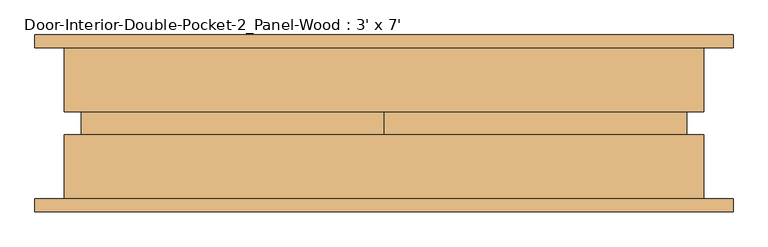
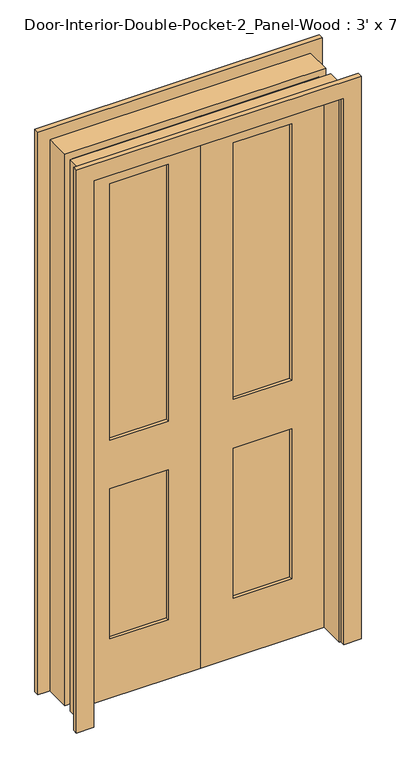
"""IFC4 building model written with IfcOpenShell, lengths in millimetres: door geometry, Door-Interior-Double-Pocket-2_Panel-Wood : 3' x 7'."""

from ifc_helpers import new_model, si_unit, frame, origin, place, context, project, spatial, polyline, outline, extrude, source, transform, mapped, element, save


def door_interior_double_pocket_2_panel_wood_3_x_7_65f9ecc5(model_context):
    return source(origin(), model_context, "Body", "SweptSolid", [
        extrude(outline(polyline([(0.0, 463.55), (0.0, 527.05), (2203.45, 527.05), (2203.45, -527.05), (0.0, -527.05), (0.0, -463.55), (2139.95, -463.55), (2139.95, 463.55), (0.0, 463.55)])), frame((0.0, 114.3, 0.0), z_axis=(0.0, 1.0, 0.0), x_axis=(0.0, 0.0, 1.0)), (0.0, 0.0, 1.0), 19.05),
        extrude(outline(polyline([(0.0, 463.55), (0.0, 527.05), (2203.45, 527.05), (2203.45, -527.05), (0.0, -527.05), (0.0, -463.55), (2139.95, -463.55), (2139.95, 463.55), (0.0, 463.55)])), frame((0.0, -133.35, 0.0), z_axis=(0.0, 1.0, 0.0), x_axis=(0.0, 0.0, 1.0)), (0.0, 0.0, 1.0), 19.05),
        extrude(outline(polyline([(2133.6, 0.0), (0.0, 0.0), (0.0, 457.2), (2133.6, 457.2), (2133.6, 0.0)]), holes=[polyline([(2014.5375, 120.65), (2014.5375, 336.55), (1009.65, 336.55), (1009.65, 120.65), (2014.5375, 120.65)]), polyline([(819.15, 120.65), (819.15, 336.55), (231.775, 336.55), (231.775, 120.65), (819.15, 120.65)])]), frame((0.0, -17.4625, 0.0), z_axis=(0.0, 1.0, 0.0), x_axis=(0.0, 0.0, 1.0)), (0.0, 0.0, 1.0), 34.925),
        extrude(outline(polyline([(336.55, -5.8208333), (120.65, -5.8208333), (120.65, 5.8208333), (336.55, 5.8208333), (336.55, -5.8208333)])), frame((0.0, 0.0, 1009.65), z_axis=(0.0, 0.0, 1.0), x_axis=(1.0, 0.0, 0.0)), (0.0, 0.0, 1.0), 1004.8875),
        extrude(outline(polyline([(336.55, -5.8208333), (120.65, -5.8208333), (120.65, 5.8208333), (336.55, 5.8208333), (336.55, -5.8208333)])), frame((0.0, 0.0, 231.775), z_axis=(0.0, 0.0, 1.0), x_axis=(1.0, 0.0, 0.0)), (0.0, 0.0, 1.0), 587.375),
        extrude(outline(polyline([(0.0, 482.6), (2159.0, 482.6), (2159.0, -482.6), (0.0, -482.6), (0.0, -457.2), (2133.6, -457.2), (2133.6, 457.2), (0.0, 457.2), (0.0, 482.6)])), frame((0.0, 17.4625, 0.0), z_axis=(0.0, 1.0, 0.0), x_axis=(0.0, 0.0, 1.0)), (0.0, 0.0, 1.0), 96.8375),
        extrude(outline(polyline([(0.0, 482.6), (2159.0, 482.6), (2159.0, -482.6), (0.0, -482.6), (0.0, -457.2), (2133.6, -457.2), (2133.6, 457.2), (0.0, 457.2), (0.0, 482.6)])), frame((0.0, -114.3, 0.0), z_axis=(0.0, 1.0, 0.0), x_axis=(0.0, 0.0, 1.0)), (0.0, 0.0, 1.0), 96.8375),
        extrude(outline(polyline([(2133.6, -457.2), (0.0, -457.2), (0.0, 0.0), (2133.6, 0.0), (2133.6, -457.2)]), holes=[polyline([(2014.5375, -336.55), (2014.5375, -120.65), (1009.65, -120.65), (1009.65, -336.55), (2014.5375, -336.55)]), polyline([(819.15, -336.55), (819.15, -120.65), (231.775, -120.65), (231.775, -336.55), (819.15, -336.55)])]), frame((0.0, -17.4625, 0.0), z_axis=(0.0, 1.0, 0.0), x_axis=(0.0, 0.0, 1.0)), (0.0, 0.0, 1.0), 34.925),
        extrude(outline(polyline([(-120.65, -5.8208333), (-336.55, -5.8208333), (-336.55, 5.8208333), (-120.65, 5.8208333), (-120.65, -5.8208333)])), frame((0.0, 0.0, 1009.65), z_axis=(0.0, 0.0, 1.0), x_axis=(1.0, 0.0, 0.0)), (0.0, 0.0, 1.0), 1004.8875),
        extrude(outline(polyline([(-120.65, -5.8208333), (-336.55, -5.8208333), (-336.55, 5.8208333), (-120.65, 5.8208333), (-120.65, -5.8208333)])), frame((0.0, 0.0, 231.775), z_axis=(0.0, 0.0, 1.0), x_axis=(1.0, 0.0, 0.0)), (0.0, 0.0, 1.0), 587.375),
    ])


if __name__ == "__main__":
    model = new_model("IFC4")
    model_context = context("Model", 3, world=origin())
    ifc_project = project(units=[si_unit("LENGTHUNIT", "METRE", prefix="MILLI")], contexts=[model_context])
    site = spatial("IfcSite", under=ifc_project)
    building = spatial("IfcBuilding", under=site)
    placement = place(None, origin())
    door_interior_double_pocket_2_panel_wood_3_x_7_shape = door_interior_double_pocket_2_panel_wood_3_x_7_65f9ecc5(model_context)
    element("IfcDoor", 1, ObjectType="Door-Interior-Double-Pocket-2_Panel-Wood : 3' x 7'", at=placement, inside=building, context=model_context, shape_type="MappedRepresentation", body=[
        mapped(door_interior_double_pocket_2_panel_wood_3_x_7_shape, transform((0.0, 0.0, 0.0), x_axis=(1.0, 0.0, 0.0), y_axis=(0.0, 1.0, 0.0), z_axis=(0.0, 0.0, 1.0))),
    ])
    save(model, "model.ifc")

# Revit data of these elements
# Type "Door-Interior-Double-Pocket-2_Panel-Wood : 3' x 7'"
#   Type Mark = "15"
#   Assembly Code = "C1020300"
#   Analytic Construction = "Wooden"
#   Top Rail = 0' - 4 11/16"
#   Thickness = 0' - 1 3/8"
#   Thermal Resistance (R) = 2.5876 (h·ft²·°F)/BTU
#   Stiles = 0' - 4 3/4"
#   Rough Width = 6' - 2"
#   Rough Height = 7' - 4 1/2"
#   Panel Width = 1' - 6"
#   Lock Rail = 0' - 7 1/2"
#   Location [instance default] = 1' - 7"
#   Height = 7' - 0"
#   Width = 3' - 0"
#   Heat Transfer Coefficient (U) = 0.3865 BTU/(h·ft²·°F)
#   Bottom Rail = 0' - 9 1/8"
#   Panel Open [instance default] = no
#   Trim Material = Cherry
#   Panel Material = Cherry
#   Frame Material = Cherry
#   Visual Light Transmittance = 0
#   Solar Heat Gain Coefficient = 0
#   Wall Closure = (empty or 0)
#   Function = (empty or 0)
# Element 1 (IfcDoor, "Door-Interior-Double-Pocket-2_Panel-Wood : 3' x 7'")
#   Materials on its faces: "Cherry"
# Materials
#   "Cherry": class "Wood", colour RGB 226 177 128, transparency 0, Description = "Prunus Serotina", Cost = 0
